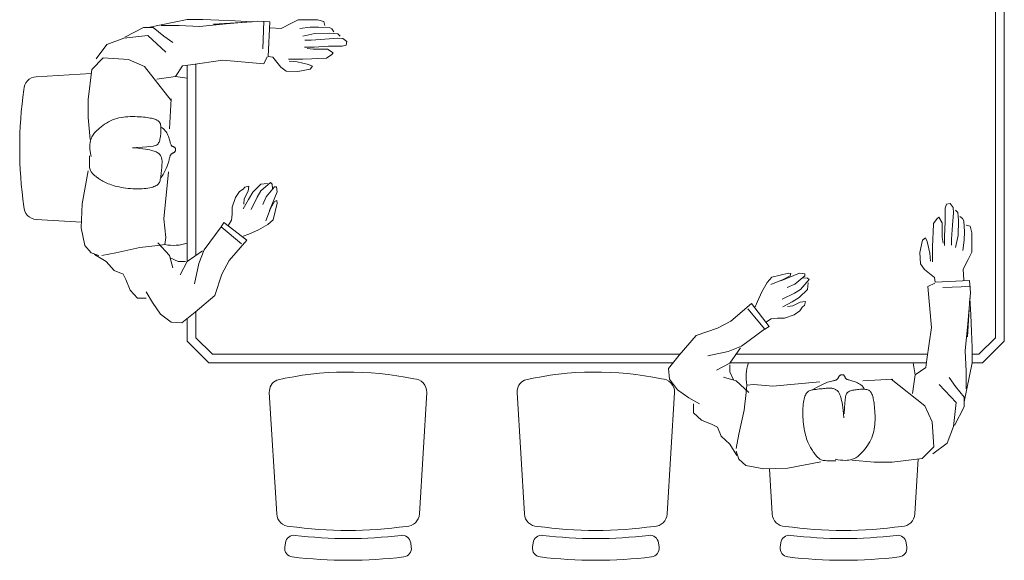
# Model space of a CAD drawing. Units: inches. Extents: x 1913 to 5309, y 1003 to 1733.
# Tile 17 of 23: x 4206 to 4274, y 1415 to 1452. Entities that reach past the tile are written whole.
import ezdxf

# ---------------------------------------------------------------- set-up
doc = ezdxf.new("R2010")
doc.units = ezdxf.units.IN
doc.layers.add('A-FURN', color=8, linetype='Continuous', lineweight=18)

# ---------------------------------------------------------------- blocks, each defined once
blk = doc.blocks.new('A$C421907B3')
for p, q in [((0.7245, 2.5796), (0.7652, 2.5876)), ((0.7652, 2.5876), (0.8209, 2.5856)), ((0.8209, 2.5856), (0.8965, 2.5714)), ((0.7017, 2.5468), (0.7079, 2.565)), ((0.7079, 2.565), (0.7245, 2.5796)), ((0.8897, 2.5609), (0.8883, 2.5594)), ((0.8911, 2.5623), (0.8897, 2.5609)), ((0.8926, 2.5635), (0.8911, 2.5623)), ((0.8941, 2.5647), (0.8926, 2.5635)), ((0.8958, 2.5657), (0.8941, 2.5647)), ((0.8976, 2.5665), (0.8958, 2.5657)), ((0.8996, 2.5672), (0.8976, 2.5665)), ((0.9018, 2.5678), (0.8996, 2.5672)), ((0.9043, 2.5682), (0.9018, 2.5678)), ((0.9071, 2.5684), (0.9043, 2.5682)), ((0.9102, 2.5686), (0.9071, 2.5684)), ((0.9137, 2.5687), (0.9102, 2.5686)), ((0.9175, 2.5687), (0.9137, 2.5687)), ((0.9217, 2.5687), (0.9175, 2.5687)), ((0.9264, 2.5687), (0.9217, 2.5687)), ((0.9314, 2.5687), (0.9264, 2.5687)), ((0.9361, 2.5662), (0.9297, 2.5647)), ((0.942, 2.5671), (0.9361, 2.5662)), ((0.9475, 2.5676), (0.942, 2.5671)), ((0.9525, 2.5677), (0.9475, 2.5676)), ((0.9571, 2.5675), (0.9525, 2.5677)), ((0.9614, 2.5669), (0.9571, 2.5675)), ((0.9652, 2.5662), (0.9614, 2.5669)), ((0.9686, 2.5653), (0.9652, 2.5662)), ((0.9684, 2.5672), (1.0195, 2.5715)), ((0.9717, 2.5643), (0.9686, 2.5653)), ((0.9745, 2.5632), (0.9717, 2.5643)), ((0.977, 2.5619), (0.9745, 2.5632)), ((0.9794, 2.5605), (0.977, 2.5619)), ((0.9818, 2.5588), (0.9794, 2.5605)), ((1.0195, 2.5715), (1.0607, 2.5715)), ((1.0607, 2.5715), (1.1301, 2.5633)), ((1.1301, 2.5633), (1.1567, 2.5368)), ((0.7038, 2.5568), (0.6875, 2.5302)), ((0.7017, 2.5405), (0.7079, 2.5077)), ((0.873, 2.5379), (0.8714, 2.5351)), ((0.8745, 2.5405), (0.873, 2.5379)), ((0.8761, 2.543), (0.8745, 2.5405)), ((0.8777, 2.5455), (0.8761, 2.543)), ((0.8792, 2.5478), (0.8777, 2.5455)), ((0.8808, 2.55), (0.8792, 2.5478)), ((0.8823, 2.5521), (0.8808, 2.55)), ((0.8839, 2.5541), (0.8823, 2.5521)), ((0.8853, 2.556), (0.8839, 2.5541)), ((0.8868, 2.5577), (0.8853, 2.556)), ((0.8883, 2.5594), (0.8868, 2.5577)), ((0.9841, 2.5568), (0.9818, 2.5588)), ((0.9865, 2.5545), (0.9841, 2.5568)), ((0.9891, 2.5519), (0.9865, 2.5545)), ((0.9918, 2.5489), (0.9891, 2.5519)), ((0.9948, 2.5455), (0.9918, 2.5489)), ((0.9978, 2.5419), (0.9948, 2.5455)), ((1.0008, 2.5379), (0.9978, 2.5419)), ((1.0037, 2.5338), (1.0008, 2.5379)), ((1.1546, 2.5531), (1.1875, 2.5285)), ((0.6875, 2.5302), (0.6672, 2.5117)), ((0.8641, 2.5181), (0.8628, 2.514)), ((0.8655, 2.522), (0.8641, 2.5181)), ((0.8669, 2.5256), (0.8655, 2.522)), ((0.8684, 2.5289), (0.8669, 2.5256)), ((0.8699, 2.5321), (0.8684, 2.5289)), ((0.8714, 2.5351), (0.8699, 2.5321)), ((1.0066, 2.5294), (1.0037, 2.5338)), ((1.0093, 2.5249), (1.0066, 2.5294)), ((1.0117, 2.5203), (1.0093, 2.5249)), ((1.0138, 2.5155), (1.0117, 2.5203)), ((1.0156, 2.5107), (1.0138, 2.5155)), ((1.1567, 2.5368), (1.153, 2.4792)), ((1.1875, 2.5285), (1.202, 2.4895)), ((0.6672, 2.5117), (0.6589, 2.4912)), ((0.7079, 2.5077), (0.7204, 2.4524)), ((0.8584, 2.4951), (0.8576, 2.49)), ((0.8594, 2.5001), (0.8584, 2.4951)), ((0.8604, 2.5049), (0.8594, 2.5001)), ((0.8616, 2.5096), (0.8604, 2.5049)), ((0.8628, 2.514), (0.8616, 2.5096)), ((1.0171, 2.5058), (1.0156, 2.5107)), ((1.0184, 2.5008), (1.0171, 2.5058)), ((1.0194, 2.4958), (1.0184, 2.5008)), ((1.0202, 2.4907), (1.0194, 2.4958)), ((0.6219, 2.4749), (0.6036, 2.4584)), ((0.6464, 2.4852), (0.6219, 2.4749)), ((0.6589, 2.4912), (0.6464, 2.4852)), ((0.8558, 2.474), (0.8554, 2.4686)), ((0.8562, 2.4794), (0.8558, 2.474)), ((0.8568, 2.4847), (0.8562, 2.4794)), ((0.8576, 2.49), (0.8568, 2.4847)), ((0.9491, 2.4609), (0.9498, 2.4698)), ((1.0208, 2.4855), (1.0202, 2.4907)), ((1.0212, 2.4802), (1.0208, 2.4855)), ((1.0214, 2.4749), (1.0212, 2.4802)), ((1.0215, 2.4696), (1.0214, 2.4749)), ((1.153, 2.4792), (1.1364, 2.4424)), ((1.202, 2.4895), (1.2083, 2.4342)), ((1.2041, 2.4875), (1.2266, 2.4445)), ((0.6036, 2.4584), (0.6036, 2.4379)), ((0.7204, 2.4524), (0.7246, 2.4114)), ((0.8552, 2.4632), (0.8551, 2.4579)), ((0.8551, 2.4579), (0.8552, 2.4527)), ((0.8554, 2.4686), (0.8552, 2.4632)), ((0.8552, 2.4527), (0.8554, 2.4476)), ((0.8554, 2.4476), (0.8557, 2.4428)), ((0.9474, 2.446), (0.9483, 2.453)), ((0.9483, 2.453), (0.9491, 2.4609)), ((0.9505, 2.4603), (0.9511, 2.447)), ((0.9511, 2.447), (0.9518, 2.4364)), ((1.0202, 2.4445), (1.0206, 2.4492)), ((1.0206, 2.4492), (1.021, 2.4541)), ((1.021, 2.4541), (1.0212, 2.4591)), ((1.0212, 2.4591), (1.0214, 2.4643)), ((1.0214, 2.4643), (1.0215, 2.4696)), ((0.6178, 2.4379), (0.5933, 2.4236)), ((0.8557, 2.4428), (0.8561, 2.4383)), ((0.8561, 2.4383), (0.8567, 2.4341)), ((0.8567, 2.4341), (0.8574, 2.4301)), ((0.8574, 2.4301), (0.8582, 2.4265)), ((0.8582, 2.4265), (0.8591, 2.4232)), ((0.9425, 2.4226), (0.9435, 2.426)), ((0.9435, 2.426), (0.9445, 2.43)), ((0.9445, 2.43), (0.9455, 2.4346)), ((0.9455, 2.4346), (0.9465, 2.4399)), ((0.9465, 2.4399), (0.9474, 2.446)), ((0.9518, 2.4364), (0.9526, 2.4283)), ((0.9526, 2.4283), (0.9535, 2.4222)), ((1.0168, 2.423), (1.0174, 2.4259)), ((1.0174, 2.4259), (1.0181, 2.429)), ((1.0181, 2.429), (1.0186, 2.4325)), ((1.0186, 2.4325), (1.0192, 2.4362)), ((1.0192, 2.4362), (1.0197, 2.4402)), ((1.0197, 2.4402), (1.0202, 2.4445)), ((1.1364, 2.4424), (1.0587, 2.3808)), ((1.2083, 2.4342), (1.1693, 2.3932)), ((1.2266, 2.4445), (1.2266, 2.422)), ((1.2447, 2.3435), (1.2266, 2.4332)), ((0.5667, 2.4051), (0.5484, 2.3805)), ((0.5933, 2.4236), (0.5667, 2.4051)), ((0.7308, 2.4114), (0.7018, 2.3846)), ((0.7246, 2.4114), (0.7267, 2.3949)), ((0.8591, 2.4232), (0.8601, 2.4202)), ((0.8601, 2.4202), (0.8612, 2.4176)), ((0.8612, 2.4176), (0.8624, 2.4152)), ((0.8624, 2.4152), (0.8637, 2.4132)), ((0.8637, 2.4132), (0.8651, 2.4114)), ((0.8651, 2.4114), (0.8666, 2.41)), ((0.8666, 2.41), (0.8682, 2.4088)), ((0.8682, 2.4088), (0.87, 2.4078)), ((0.87, 2.4078), (0.872, 2.407)), ((0.872, 2.407), (0.8742, 2.4063)), ((0.8742, 2.4063), (0.8767, 2.4058)), ((0.8767, 2.4058), (0.8794, 2.4052)), ((0.8794, 2.4052), (0.8824, 2.4048)), ((0.8801, 2.4042), (0.8884, 2.3992)), ((0.8824, 2.4048), (0.8857, 2.4043)), ((0.8857, 2.4043), (0.8891, 2.4039)), ((0.8891, 2.4039), (0.8925, 2.4035)), ((0.8925, 2.4035), (0.896, 2.4031)), ((0.896, 2.4031), (0.8995, 2.4027)), ((0.8995, 2.4027), (0.9028, 2.4024)), ((0.9028, 2.4024), (0.9059, 2.4022)), ((0.9059, 2.4022), (0.9088, 2.4019)), ((0.9088, 2.4019), (0.9114, 2.4018)), ((0.9114, 2.4018), (0.9138, 2.4016)), ((0.9182, 2.4016), (0.9201, 2.4017)), ((0.9201, 2.4017), (0.9219, 2.4019)), ((0.9219, 2.4019), (0.9237, 2.4022)), ((0.9237, 2.4022), (0.9254, 2.4026)), ((0.9254, 2.4026), (0.927, 2.4031)), ((0.927, 2.4031), (0.9286, 2.4037)), ((0.9286, 2.4037), (0.9301, 2.4044)), ((0.9301, 2.4044), (0.9315, 2.4052)), ((0.9315, 2.4052), (0.9329, 2.406)), ((0.9329, 2.406), (0.9341, 2.4069)), ((0.9341, 2.4069), (0.9353, 2.4079)), ((0.9353, 2.4079), (0.9363, 2.409)), ((0.9363, 2.409), (0.9373, 2.4102)), ((0.9373, 2.4102), (0.9382, 2.4116)), ((0.9382, 2.4116), (0.9391, 2.4131)), ((0.9391, 2.4131), (0.9399, 2.415)), ((0.9399, 2.415), (0.9408, 2.4171)), ((0.9408, 2.4171), (0.9416, 2.4196)), ((0.9416, 2.4196), (0.9425, 2.4226)), ((0.9535, 2.4222), (0.9546, 2.4177)), ((0.9546, 2.4177), (0.9558, 2.4146)), ((0.9558, 2.4146), (0.9572, 2.4124)), ((0.9572, 2.4124), (0.9588, 2.4109)), ((0.9588, 2.4109), (0.9606, 2.4096)), ((0.9606, 2.4096), (0.9626, 2.4086)), ((0.9626, 2.4086), (0.9647, 2.4077)), ((0.9647, 2.4077), (0.9671, 2.407)), ((0.9671, 2.407), (0.9696, 2.4064)), ((0.9696, 2.4064), (0.9722, 2.406)), ((0.9722, 2.406), (0.9751, 2.4055)), ((0.9751, 2.4055), (0.9781, 2.4052)), ((0.9781, 2.4052), (0.9812, 2.4048)), ((0.9812, 2.4048), (0.9844, 2.4045)), ((0.9844, 2.4045), (0.9877, 2.4043)), ((0.9877, 2.4043), (0.9909, 2.4041)), ((0.9909, 2.4041), (0.9941, 2.4041)), ((0.994, 2.3993), (0.9965, 2.4026)), ((0.9941, 2.4041), (0.9971, 2.4042)), ((0.9971, 2.4042), (0.9999, 2.4044)), ((0.9999, 2.4044), (1.0025, 2.4049)), ((1.0025, 2.4049), (1.0047, 2.4055)), ((1.0047, 2.4055), (1.0067, 2.4064)), ((1.0067, 2.4064), (1.0085, 2.4075)), ((1.0085, 2.4075), (1.01, 2.4087)), ((1.01, 2.4087), (1.0113, 2.4102)), ((1.0113, 2.4102), (1.0124, 2.4119)), ((1.0124, 2.4119), (1.0135, 2.4137)), ((1.0135, 2.4137), (1.0144, 2.4158)), ((1.0144, 2.4158), (1.0152, 2.418)), ((1.0152, 2.418), (1.016, 2.4204)), ((1.016, 2.4204), (1.0168, 2.423)), ((1.1077, 2.4136), (1.114, 2.3706)), ((1.2266, 2.422), (1.2062, 2.3974)), ((1.2308, 2.3624), (1.2308, 2.4035)), ((0.5484, 2.3805), (0.5463, 2.356)), ((0.7018, 2.3846), (0.6731, 2.3766)), ((0.6876, 2.3643), (0.6959, 2.3826)), ((0.7267, 2.3949), (0.7429, 2.3929)), ((0.7429, 2.3929), (0.7861, 2.3972)), ((0.7861, 2.3972), (0.8946, 2.387)), ((0.8884, 2.3992), (0.8957, 2.3952)), ((0.8957, 2.3952), (0.9019, 2.3921)), ((0.9019, 2.3921), (0.9073, 2.3897)), ((0.9073, 2.3897), (0.9119, 2.3881)), ((0.9119, 2.3881), (0.9157, 2.3869)), ((0.9138, 2.4016), (0.9161, 2.4016)), ((0.9157, 2.3869), (0.919, 2.386)), ((0.9161, 2.4016), (0.9182, 2.4016)), ((0.919, 2.386), (0.9217, 2.3854)), ((0.9217, 2.3854), (0.924, 2.3849)), ((0.924, 2.3849), (0.926, 2.3844)), ((0.926, 2.3844), (0.9277, 2.384)), ((0.9277, 2.384), (0.929, 2.3837)), ((0.929, 2.3837), (0.9302, 2.3833)), ((0.9302, 2.3833), (0.9312, 2.383)), ((0.9312, 2.383), (0.932, 2.3826)), ((0.932, 2.3826), (0.9327, 2.3823)), ((0.9327, 2.3823), (0.9334, 2.3818)), ((0.9334, 2.3818), (0.934, 2.3813)), ((0.934, 2.3813), (0.9346, 2.3808)), ((0.9346, 2.3808), (0.9351, 2.3803)), ((0.9351, 2.3803), (0.9356, 2.3797)), ((0.9356, 2.3797), (0.936, 2.379)), ((0.9533, 2.3785), (0.9536, 2.379)), ((0.9536, 2.379), (0.954, 2.3796)), ((0.954, 2.3796), (0.9546, 2.3801)), ((0.9546, 2.3801), (0.9554, 2.3805)), ((0.9554, 2.3805), (0.9564, 2.381)), ((0.9564, 2.381), (0.9577, 2.3815)), ((0.9577, 2.3815), (0.9593, 2.382)), ((0.9593, 2.382), (0.9611, 2.3826)), ((0.9611, 2.3826), (0.9632, 2.3832)), ((0.9632, 2.3832), (0.9655, 2.3838)), ((0.9655, 2.3838), (0.9679, 2.3845)), ((0.9679, 2.3845), (0.9705, 2.3853)), ((0.9705, 2.3853), (0.9731, 2.3861)), ((0.9731, 2.3861), (0.9757, 2.387)), ((0.9757, 2.387), (0.9784, 2.388)), ((0.9784, 2.388), (0.9811, 2.3892)), ((0.9811, 2.3892), (0.9837, 2.3905)), ((0.9837, 2.3905), (0.9863, 2.3922)), ((0.9863, 2.3922), (0.9889, 2.3941)), ((0.9889, 2.3941), (0.9915, 2.3965)), ((0.9915, 2.3965), (0.994, 2.3993)), ((0.9931, 2.3848), (1.0625, 2.3808)), ((1.2062, 2.3974), (1.1917, 2.3769)), ((0.6569, 2.3601), (0.6876, 2.3438)), ((0.6876, 2.3478), (0.6876, 2.3643)), ((0.936, 2.379), (0.9365, 2.3783)), ((0.9365, 2.3783), (0.9369, 2.3776)), ((0.9369, 2.3776), (0.9372, 2.3769)), ((0.9372, 2.3769), (0.9376, 2.3761)), ((0.9376, 2.3761), (0.938, 2.3753)), ((0.938, 2.3753), (0.9384, 2.3746)), ((0.9384, 2.3746), (0.9389, 2.3738)), ((0.9389, 2.3738), (0.9395, 2.3731)), ((0.9395, 2.3731), (0.9401, 2.3725)), ((0.9401, 2.3725), (0.9408, 2.3719)), ((0.9408, 2.3719), (0.9417, 2.3714)), ((0.9417, 2.3714), (0.9426, 2.371)), ((0.9426, 2.371), (0.9437, 2.3707)), ((0.9437, 2.3707), (0.9447, 2.3706)), ((0.9447, 2.3706), (0.9458, 2.3705)), ((0.9458, 2.3705), (0.9468, 2.3706)), ((0.9468, 2.3706), (0.9478, 2.3708)), ((0.9478, 2.3708), (0.9487, 2.3712)), ((0.9487, 2.3712), (0.9494, 2.3717)), ((0.9494, 2.3717), (0.9501, 2.3723)), ((0.9501, 2.3723), (0.9507, 2.3731)), ((0.9507, 2.3731), (0.9512, 2.3739)), ((0.9512, 2.3739), (0.9517, 2.3747)), ((0.9517, 2.3747), (0.9521, 2.3755)), ((0.9521, 2.3755), (0.9524, 2.3764)), ((0.9524, 2.3764), (0.9527, 2.3771)), ((0.9527, 2.3771), (0.953, 2.3778)), ((0.953, 2.3778), (0.9533, 2.3785)), ((1.114, 2.3706), (1.1095, 2.3436)), ((1.114, 2.3706), (1.1385, 2.3544)), ((1.2287, 2.3154), (1.2308, 2.3624)), ((0.5463, 2.356), (0.5709, 2.3252)), ((0.6876, 2.3438), (0.7122, 2.3088)), ((1.1385, 2.3544), (1.1406, 2.3358)), ((1.1406, 2.3358), (1.151, 2.262)), ((0.5709, 2.3252), (0.6099, 2.2802)), ((0.6835, 2.317), (0.6365, 2.3273)), ((0.7143, 2.3048), (0.6835, 2.317)), ((1.235, 2.2538), (1.2287, 2.3154)), ((0.7674, 2.2656), (0.7143, 2.3048)), ((0.6099, 2.2802), (0.659, 2.2637)), ((0.7288, 2.2187), (0.7675, 2.2658)), ((0.7675, 2.2658), (0.7779, 2.2598)), ((0.659, 2.2637), (0.6898, 2.2475)), ((0.6898, 2.2475), (0.7368, 2.2065)), ((0.7779, 2.2598), (0.7368, 2.2065)), ((0.7716, 2.2487), (0.7827, 2.2421)), ((1.151, 2.262), (1.1428, 2.1677)), ((1.2413, 2.1822), (1.235, 2.2538)), ((0.7827, 2.2421), (0.7969, 2.2406)), ((0.7969, 2.2406), (0.8131, 2.2406)), ((0.8131, 2.2406), (0.8354, 2.2325)), ((0.8354, 2.2325), (0.8487, 2.2236)), ((0.8487, 2.2236), (0.8546, 2.2147)), ((0.7509, 2.2021), (0.7458, 2.2146)), ((0.7606, 2.1798), (0.7509, 2.2021)), ((0.8094, 2.2146), (0.8309, 2.2028)), ((0.8324, 2.2124), (0.8198, 2.2132)), ((0.8309, 2.2028), (0.8472, 2.1925)), ((0.8494, 2.2036), (0.8324, 2.2124)), ((0.8613, 2.2021), (0.8494, 2.2036)), ((0.8546, 2.2147), (0.859, 2.211)), ((0.859, 2.211), (0.8613, 2.2021)), ((0.7732, 2.1583), (0.7606, 2.1798)), ((0.8079, 2.1969), (0.8361, 2.1828)), ((0.8361, 2.1828), (0.8502, 2.1747)), ((0.8472, 2.1925), (0.8658, 2.1747)), ((1.2392, 2.1535), (1.2413, 2.1822)), ((0.7835, 2.1457), (0.7732, 2.1583)), ((0.7814, 2.1628), (0.8102, 2.1517)), ((0.848, 2.1369), (0.805, 2.1547)), ((0.8191, 2.1695), (0.8369, 2.1621)), ((0.8369, 2.1621), (0.8599, 2.1429)), ((0.8502, 2.1747), (0.8695, 2.1518)), ((0.8658, 2.1747), (0.8672, 2.1591)), ((1.1428, 2.1677), (1.159, 2.1597)), ((1.1595, 2.1573), (1.158, 2.1467)), ((1.1595, 2.1573), (1.2392, 2.1535)), ((1.1777, 2.1697), (1.2413, 2.1677)), ((1.226, 2.1528), (1.2245, 2.1279)), ((0.8221, 2.1369), (0.7835, 2.1457)), ((0.8102, 2.1517), (0.8257, 2.1428)), ((0.828, 2.1376), (0.8221, 2.1369)), ((0.8257, 2.1428), (0.828, 2.1376)), ((0.8599, 2.1384), (0.848, 2.1369)), ((0.8658, 2.1481), (0.8561, 2.1473)), ((0.8599, 2.1429), (0.8599, 2.1384)), ((0.8695, 2.1518), (0.8658, 2.1481)), ((1.158, 2.1467), (1.1354, 2.1286)), ((1.1263, 2.1158), (1.1248, 2.0893)), ((1.1354, 2.1286), (1.1263, 2.1158)), ((1.1474, 2.0909), (1.149, 2.1089)), ((1.1535, 2.1105), (1.1536, 2.078)), ((1.2245, 2.1279), (1.2358, 2.1052)), ((1.1248, 2.0893), (1.1308, 2.0606)), ((1.1414, 2.0644), (1.1474, 2.0909)), ((1.2238, 2.0848), (1.2269, 2.0606)), ((1.2358, 2.1052), (1.2442, 2.0886)), ((1.2442, 2.0886), (1.2442, 2.0441)), ((1.1377, 2.0553), (1.1414, 2.0644)), ((1.1536, 2.078), (1.1543, 2.0568)), ((1.1762, 2.0539), (1.1784, 2.0674)), ((1.1815, 2.0735), (1.1815, 2.0516)), ((1.1974, 2.0584), (1.1974, 2.0727)), ((1.2064, 2.078), (1.2125, 2.0501)), ((1.1308, 2.0606), (1.1377, 2.0553)), ((1.1543, 2.0568), (1.1551, 2.0432)), ((1.1551, 2.0432), (1.1558, 2.0229)), ((1.1762, 2.0357), (1.1762, 2.0539)), ((1.1815, 2.0516), (1.1831, 2.0183)), ((1.1996, 2.0267), (1.1974, 2.0584)), ((1.2125, 2.0501), (1.2132, 2.0154)), ((1.2276, 2.0418), (1.2261, 2.0161)), ((1.2269, 2.0606), (1.2276, 2.0418)), ((1.2442, 2.0441), (1.2404, 2.029)), ((1.1558, 2.0229), (1.1641, 2.0108)), ((1.168, 2.0077), (1.1762, 2.0206)), ((1.1762, 2.0206), (1.1762, 2.0357)), ((1.1831, 2.0183), (1.1831, 1.9874)), ((1.2019, 1.9979), (1.1996, 2.0267)), ((1.2404, 2.029), (1.2314, 2.0267)), ((1.1641, 2.0108), (1.168, 2.0077)), ((1.2012, 1.9859), (1.2019, 1.9979)), ((1.2117, 1.9972), (1.2064, 1.9919)), ((1.2132, 2.0154), (1.2117, 1.9972)), ((1.223, 2.0108), (1.2163, 2.0063)), ((1.2261, 2.0161), (1.223, 2.0108)), ((1.1831, 1.9874), (1.186, 1.9783)), ((1.186, 1.9783), (1.1944, 1.9768)), ((1.1944, 1.9768), (1.2012, 1.9859)), ((0.3928, 1.2157), (0.4173, 1.234)), ((0.4173, 1.234), (0.4418, 1.2361)), ((0.4418, 1.2361), (0.4726, 1.2115)), ((0.3742, 1.1891), (0.3928, 1.2157)), ((0.4726, 1.2115), (0.5176, 1.1724)), ((0.3229, 1.1605), (0.3394, 1.1788)), ((0.3394, 1.1788), (0.36, 1.1787)), ((0.36, 1.1646), (0.3742, 1.1891)), ((0.3126, 1.1359), (0.3229, 1.1605)), ((0.5176, 1.1724), (0.5341, 1.1234)), ((0.3066, 1.1235), (0.3126, 1.1359)), ((0.4808, 1.0989), (0.4706, 1.1459)), ((0.2676, 1.0948), (0.2861, 1.1152)), ((0.2861, 1.1152), (0.3066, 1.1235)), ((0.4378, 1.1255), (0.454, 1.0947)), ((0.5341, 1.1234), (0.5503, 1.0926)), ((0.241, 1.0786), (0.2676, 1.0948)), ((0.4132, 1.0806), (0.4212, 1.1093)), ((0.4335, 1.0947), (0.4152, 1.0865)), ((0.45, 1.0947), (0.4335, 1.0947)), ((0.454, 1.0947), (0.489, 1.0702)), ((0.493, 1.0681), (0.4808, 1.0989)), ((0.5503, 1.0926), (0.5914, 1.0456)), ((0.2328, 1.0745), (0.2183, 1.0579)), ((0.2511, 1.0807), (0.2328, 1.0745)), ((0.2573, 1.0807), (0.2901, 1.0744)), ((0.2901, 1.0744), (0.3454, 1.062)), ((0.3864, 1.0516), (0.4132, 1.0806)), ((0.5322, 1.015), (0.493, 1.0681)), ((0.2183, 1.0579), (0.2102, 1.0171)), ((0.3454, 1.062), (0.3864, 1.0578)), ((0.3864, 1.0578), (0.4029, 1.0557)), ((0.4029, 1.0557), (0.4049, 1.0395)), ((0.5791, 1.0535), (0.532, 1.0149)), ((0.538, 1.0045), (0.5914, 1.0456)), ((0.4049, 1.0395), (0.4006, 0.9963)), ((0.5958, 1.0315), (0.5832, 1.0366)), ((0.618, 1.0218), (0.5958, 1.0315)), ((0.6395, 1.0092), (0.618, 1.0218)), ((0.2102, 1.0171), (0.2122, 0.9615)), ((0.532, 1.0149), (0.538, 1.0045)), ((0.5491, 1.0108), (0.5557, 0.9996)), ((0.5557, 0.9996), (0.5572, 0.9855)), ((0.635, 1.001), (0.6461, 0.9722)), ((0.6521, 0.9988), (0.6395, 1.0092)), ((0.6609, 0.9603), (0.6521, 0.9988)), ((0.4006, 0.9963), (0.4108, 0.8878)), ((0.5572, 0.9855), (0.5572, 0.9693)), ((0.6009, 0.9744), (0.615, 0.9462)), ((0.6609, 0.9344), (0.6432, 0.9774)), ((0.2122, 0.9615), (0.2264, 0.8858)), ((0.5572, 0.9693), (0.5653, 0.947)), ((0.5832, 0.9729), (0.595, 0.9515)), ((0.5854, 0.9499), (0.5846, 0.9626)), ((0.6283, 0.9633), (0.6357, 0.9455)), ((0.6461, 0.9722), (0.655, 0.9566)), ((0.655, 0.9566), (0.6602, 0.9544)), ((0.6602, 0.9544), (0.6609, 0.9603)), ((0.5653, 0.947), (0.5742, 0.9337)), ((0.5742, 0.9337), (0.5832, 0.9278)), ((0.5942, 0.933), (0.5854, 0.9499)), ((0.5957, 0.9211), (0.5942, 0.933)), ((0.595, 0.9515), (0.6053, 0.9352)), ((0.6053, 0.9352), (0.6232, 0.9166)), ((0.615, 0.9462), (0.6232, 0.9322)), ((0.6232, 0.9322), (0.6461, 0.9129)), ((0.6357, 0.9455), (0.655, 0.9225)), ((0.6594, 0.9225), (0.6609, 0.9344)), ((0.2548, 0.9063), (0.2573, 0.9078)), ((0.2573, 0.9078), (0.26, 0.9094)), ((0.26, 0.9094), (0.2628, 0.911)), ((0.2628, 0.911), (0.2657, 0.9125)), ((0.2657, 0.9125), (0.2689, 0.914)), ((0.2689, 0.914), (0.2723, 0.9155)), ((0.2723, 0.9155), (0.2759, 0.9169)), ((0.2759, 0.9169), (0.2797, 0.9183)), ((0.2797, 0.9183), (0.2839, 0.9196)), ((0.2839, 0.9196), (0.2883, 0.9208)), ((0.2883, 0.9208), (0.2929, 0.922)), ((0.2929, 0.922), (0.2977, 0.923)), ((0.2977, 0.923), (0.3027, 0.924)), ((0.3027, 0.924), (0.3078, 0.9248)), ((0.3078, 0.9248), (0.3131, 0.9255)), ((0.3131, 0.9255), (0.3184, 0.9261)), ((0.3184, 0.9261), (0.3238, 0.9266)), ((0.3238, 0.9266), (0.3293, 0.927)), ((0.3293, 0.927), (0.3347, 0.9272)), ((0.3347, 0.9272), (0.34, 0.9272)), ((0.34, 0.9272), (0.3452, 0.9272)), ((0.3452, 0.9272), (0.3502, 0.927)), ((0.3502, 0.927), (0.355, 0.9267)), ((0.355, 0.9267), (0.3595, 0.9262)), ((0.3595, 0.9262), (0.3638, 0.9257)), ((0.3638, 0.9257), (0.3677, 0.925)), ((0.3677, 0.925), (0.3713, 0.9242)), ((0.3713, 0.9242), (0.3746, 0.9233)), ((0.3746, 0.9233), (0.3776, 0.9223)), ((0.3776, 0.9223), (0.3803, 0.9212)), ((0.3803, 0.9212), (0.3826, 0.92)), ((0.3826, 0.92), (0.3847, 0.9187)), ((0.3847, 0.9187), (0.3864, 0.9173)), ((0.3864, 0.9173), (0.3878, 0.9158)), ((0.3878, 0.9158), (0.389, 0.9142)), ((0.389, 0.9142), (0.39, 0.9123)), ((0.39, 0.9123), (0.3908, 0.9104)), ((0.3908, 0.9104), (0.3915, 0.9081)), ((0.3915, 0.9081), (0.3921, 0.9057)), ((0.5832, 0.9278), (0.5869, 0.9233)), ((0.5869, 0.9233), (0.5957, 0.9211)), ((0.6232, 0.9166), (0.6387, 0.9151)), ((0.6461, 0.9129), (0.6498, 0.9166)), ((0.6498, 0.9166), (0.6506, 0.9263)), ((0.655, 0.9225), (0.6594, 0.9225)), ((0.2306, 0.8828), (0.2313, 0.8848)), ((0.2313, 0.8848), (0.2322, 0.8866)), ((0.2322, 0.8866), (0.2332, 0.8883)), ((0.2332, 0.8883), (0.2343, 0.8898)), ((0.2343, 0.8898), (0.2356, 0.8913)), ((0.2356, 0.8913), (0.237, 0.8927)), ((0.237, 0.8927), (0.2385, 0.8941)), ((0.2385, 0.8941), (0.2401, 0.8956)), ((0.2401, 0.8956), (0.2419, 0.897)), ((0.2419, 0.897), (0.2437, 0.8985)), ((0.2437, 0.8985), (0.2457, 0.9)), ((0.2457, 0.9), (0.2478, 0.9016)), ((0.2478, 0.9016), (0.25, 0.9031)), ((0.25, 0.9031), (0.2524, 0.9047)), ((0.2524, 0.9047), (0.2548, 0.9063)), ((0.3921, 0.9057), (0.3926, 0.903)), ((0.3926, 0.903), (0.3931, 0.8999)), ((0.3931, 0.8999), (0.3935, 0.8967)), ((0.3935, 0.8967), (0.394, 0.8933)), ((0.3936, 0.9023), (0.3986, 0.894)), ((0.394, 0.8933), (0.3944, 0.8898)), ((0.3944, 0.8898), (0.3947, 0.8863)), ((0.3947, 0.8863), (0.3951, 0.8829)), ((0.3986, 0.894), (0.4026, 0.8867)), ((0.4026, 0.8867), (0.4057, 0.8804)), ((0.2291, 0.8687), (0.2292, 0.8722)), ((0.2291, 0.8649), (0.2291, 0.8687)), ((0.2291, 0.8607), (0.2291, 0.8649)), ((0.2292, 0.8722), (0.2294, 0.8753)), ((0.2294, 0.8753), (0.2297, 0.8781)), ((0.2297, 0.8781), (0.2301, 0.8806)), ((0.2301, 0.8806), (0.2306, 0.8828)), ((0.3951, 0.8829), (0.3954, 0.8796)), ((0.3954, 0.8796), (0.3957, 0.8765)), ((0.3957, 0.8765), (0.3959, 0.8736)), ((0.3959, 0.8736), (0.3961, 0.871)), ((0.3961, 0.8623), (0.3959, 0.8604)), ((0.3961, 0.871), (0.3962, 0.8685)), ((0.3962, 0.8642), (0.3961, 0.8623)), ((0.3962, 0.8685), (0.3962, 0.8663)), ((0.3962, 0.8663), (0.3962, 0.8642)), ((0.4057, 0.8804), (0.4081, 0.8751)), ((0.4081, 0.8751), (0.4098, 0.8705)), ((0.4098, 0.8705), (0.411, 0.8667)), ((0.411, 0.8667), (0.4118, 0.8634)), ((0.4118, 0.8634), (0.4124, 0.8607)), ((0.2291, 0.856), (0.2291, 0.8607)), ((0.2291, 0.8509), (0.2291, 0.856)), ((0.2302, 0.8349), (0.2307, 0.8404)), ((0.2307, 0.8404), (0.2316, 0.8463)), ((0.2316, 0.8463), (0.2331, 0.8527)), ((0.3718, 0.8389), (0.3678, 0.8379)), ((0.3752, 0.8398), (0.3718, 0.8389)), ((0.3782, 0.8407), (0.3752, 0.8398)), ((0.3807, 0.8416), (0.3782, 0.8407)), ((0.3829, 0.8425), (0.3807, 0.8416)), ((0.3847, 0.8433), (0.3829, 0.8425)), ((0.3863, 0.8442), (0.3847, 0.8433)), ((0.3876, 0.8451), (0.3863, 0.8442)), ((0.3888, 0.846), (0.3876, 0.8451)), ((0.3899, 0.8471), (0.3888, 0.846)), ((0.3909, 0.8482), (0.3899, 0.8471)), ((0.3918, 0.8495), (0.3909, 0.8482)), ((0.3927, 0.8508), (0.3918, 0.8495)), ((0.3934, 0.8523), (0.3927, 0.8508)), ((0.3941, 0.8538), (0.3934, 0.8523)), ((0.3947, 0.8553), (0.3941, 0.8538)), ((0.3952, 0.857), (0.3947, 0.8553)), ((0.3956, 0.8587), (0.3952, 0.857)), ((0.3959, 0.8604), (0.3956, 0.8587)), ((0.4124, 0.8607), (0.4129, 0.8583)), ((0.4129, 0.8583), (0.4134, 0.8564)), ((0.4134, 0.8564), (0.4138, 0.8547)), ((0.4138, 0.8547), (0.4141, 0.8533)), ((0.4141, 0.8533), (0.4145, 0.8522)), ((0.4145, 0.8522), (0.4148, 0.8512)), ((0.4148, 0.8512), (0.4152, 0.8504)), ((0.4152, 0.8504), (0.4156, 0.8497)), ((0.4156, 0.8497), (0.416, 0.849)), ((0.416, 0.849), (0.4165, 0.8484)), ((0.4165, 0.8484), (0.417, 0.8478)), ((0.417, 0.8478), (0.4176, 0.8473)), ((0.4176, 0.8473), (0.4182, 0.8468)), ((0.4182, 0.8468), (0.4188, 0.8463)), ((0.4188, 0.8463), (0.4195, 0.8459)), ((0.4195, 0.8459), (0.4202, 0.8455)), ((0.4202, 0.8455), (0.4209, 0.8451)), ((0.4209, 0.8451), (0.4217, 0.8448)), ((0.4217, 0.8448), (0.4225, 0.8444)), ((0.4225, 0.8444), (0.4233, 0.8439)), ((0.4233, 0.8439), (0.424, 0.8435)), ((0.424, 0.8435), (0.4247, 0.8429)), ((0.4247, 0.8429), (0.4253, 0.8423)), ((0.4253, 0.8423), (0.4259, 0.8415)), ((0.4259, 0.8415), (0.4264, 0.8407)), ((0.4264, 0.8407), (0.4268, 0.8397)), ((0.4268, 0.8397), (0.4271, 0.8387)), ((0.4271, 0.8387), (0.4273, 0.8377)), ((0.2301, 0.8299), (0.2302, 0.8349)), ((0.2304, 0.8252), (0.2301, 0.8299)), ((0.2309, 0.821), (0.2304, 0.8252)), ((0.2316, 0.8172), (0.2309, 0.821)), ((0.2325, 0.8138), (0.2316, 0.8172)), ((0.3369, 0.8333), (0.328, 0.8326)), ((0.3448, 0.8341), (0.3369, 0.8333)), ((0.3375, 0.8319), (0.3508, 0.8313)), ((0.3518, 0.835), (0.3448, 0.8341)), ((0.3508, 0.8313), (0.3614, 0.8306)), ((0.3579, 0.8359), (0.3518, 0.835)), ((0.3632, 0.8369), (0.3579, 0.8359)), ((0.3614, 0.8306), (0.3695, 0.8298)), ((0.3678, 0.8379), (0.3632, 0.8369)), ((0.3695, 0.8298), (0.3757, 0.8289)), ((0.3757, 0.8289), (0.3801, 0.8278)), ((0.3801, 0.8278), (0.3832, 0.8265)), ((0.3832, 0.8265), (0.3854, 0.8251)), ((0.3854, 0.8251), (0.3869, 0.8235)), ((0.3869, 0.8235), (0.3882, 0.8218)), ((0.3882, 0.8218), (0.3892, 0.8198)), ((0.3892, 0.8198), (0.3901, 0.8176)), ((0.3901, 0.8176), (0.3908, 0.8153)), ((0.414, 0.8169), (0.4133, 0.8145)), ((0.4147, 0.8192), (0.414, 0.8169)), ((0.4152, 0.8213), (0.4147, 0.8192)), ((0.4158, 0.8231), (0.4152, 0.8213)), ((0.4163, 0.8247), (0.4158, 0.8231)), ((0.4168, 0.826), (0.4163, 0.8247)), ((0.4173, 0.827), (0.4168, 0.826)), ((0.4178, 0.8277), (0.4173, 0.827)), ((0.4183, 0.8283), (0.4178, 0.8277)), ((0.4188, 0.8288), (0.4183, 0.8283)), ((0.4194, 0.8291), (0.4188, 0.8288)), ((0.42, 0.8294), (0.4194, 0.8291)), ((0.4207, 0.8297), (0.42, 0.8294)), ((0.4215, 0.83), (0.4207, 0.8297)), ((0.4223, 0.8303), (0.4215, 0.83)), ((0.4231, 0.8307), (0.4223, 0.8303)), ((0.424, 0.8311), (0.4231, 0.8307)), ((0.4248, 0.8316), (0.424, 0.8311)), ((0.4255, 0.8322), (0.4248, 0.8316)), ((0.4261, 0.8329), (0.4255, 0.8322)), ((0.4267, 0.8337), (0.4261, 0.8329)), ((0.427, 0.8346), (0.4267, 0.8337)), ((0.4272, 0.8356), (0.427, 0.8346)), ((0.4273, 0.8366), (0.4272, 0.8356)), ((0.4273, 0.8377), (0.4273, 0.8366)), ((0.2306, 0.814), (0.2263, 0.7628)), ((0.2335, 0.8107), (0.2325, 0.8138)), ((0.2346, 0.8079), (0.2335, 0.8107)), ((0.2359, 0.8053), (0.2346, 0.8079)), ((0.2374, 0.8029), (0.2359, 0.8053)), ((0.2391, 0.8006), (0.2374, 0.8029)), ((0.241, 0.7983), (0.2391, 0.8006)), ((0.2433, 0.7958), (0.241, 0.7983)), ((0.246, 0.7933), (0.2433, 0.7958)), ((0.249, 0.7905), (0.246, 0.7933)), ((0.3908, 0.8153), (0.3914, 0.8128)), ((0.3914, 0.8128), (0.3919, 0.8101)), ((0.3919, 0.8101), (0.3923, 0.8073)), ((0.3923, 0.8073), (0.3926, 0.8043)), ((0.3926, 0.8043), (0.393, 0.8012)), ((0.393, 0.8012), (0.3933, 0.7979)), ((0.3933, 0.7979), (0.3936, 0.7947)), ((0.3936, 0.7947), (0.3937, 0.7915)), ((0.4037, 0.7935), (0.4014, 0.7909)), ((0.4057, 0.796), (0.4037, 0.7935)), ((0.4073, 0.7987), (0.4057, 0.796)), ((0.4087, 0.8013), (0.4073, 0.7987)), ((0.4098, 0.804), (0.4087, 0.8013)), ((0.4108, 0.8066), (0.4098, 0.804)), ((0.4117, 0.8093), (0.4108, 0.8066)), ((0.4126, 0.8119), (0.4117, 0.8093)), ((0.4133, 0.8145), (0.4126, 0.8119)), ((0.2523, 0.7876), (0.249, 0.7905)), ((0.256, 0.7846), (0.2523, 0.7876)), ((0.2599, 0.7816), (0.256, 0.7846)), ((0.264, 0.7786), (0.2599, 0.7816)), ((0.2684, 0.7758), (0.264, 0.7786)), ((0.2729, 0.7731), (0.2684, 0.7758)), ((0.2776, 0.7707), (0.2729, 0.7731)), ((0.2823, 0.7686), (0.2776, 0.7707)), ((0.3876, 0.7711), (0.386, 0.7699)), ((0.3891, 0.7724), (0.3876, 0.7711)), ((0.3904, 0.7739), (0.3891, 0.7724)), ((0.3914, 0.7756), (0.3904, 0.7739)), ((0.3923, 0.7776), (0.3914, 0.7756)), ((0.393, 0.7799), (0.3923, 0.7776)), ((0.3934, 0.7825), (0.393, 0.7799)), ((0.3937, 0.7853), (0.3934, 0.7825)), ((0.3937, 0.7915), (0.3938, 0.7883)), ((0.3938, 0.7883), (0.3937, 0.7853)), ((0.3986, 0.7884), (0.3953, 0.7859)), ((0.4014, 0.7909), (0.3986, 0.7884)), ((0.413, 0.7893), (0.417, 0.7199)), ((0.2263, 0.7628), (0.2263, 0.7217)), ((0.2871, 0.7668), (0.2823, 0.7686)), ((0.292, 0.7652), (0.2871, 0.7668)), ((0.297, 0.764), (0.292, 0.7652)), ((0.302, 0.7629), (0.297, 0.764)), ((0.3071, 0.7621), (0.302, 0.7629)), ((0.3123, 0.7616), (0.3071, 0.7621)), ((0.3176, 0.7612), (0.3123, 0.7616)), ((0.3229, 0.7609), (0.3176, 0.7612)), ((0.3282, 0.7609), (0.3229, 0.7609)), ((0.3335, 0.7609), (0.3282, 0.7609)), ((0.3387, 0.7611), (0.3335, 0.7609)), ((0.3438, 0.7614), (0.3387, 0.7611)), ((0.3486, 0.7618), (0.3438, 0.7614)), ((0.3533, 0.7622), (0.3486, 0.7618)), ((0.3576, 0.7627), (0.3533, 0.7622)), ((0.3617, 0.7632), (0.3576, 0.7627)), ((0.3654, 0.7637), (0.3617, 0.7632)), ((0.3688, 0.7643), (0.3654, 0.7637)), ((0.3719, 0.7649), (0.3688, 0.7643)), ((0.3748, 0.7656), (0.3719, 0.7649)), ((0.3774, 0.7663), (0.3748, 0.7656)), ((0.3799, 0.7671), (0.3774, 0.7663)), ((0.3821, 0.768), (0.3799, 0.7671)), ((0.3841, 0.7689), (0.3821, 0.768)), ((0.386, 0.7699), (0.3841, 0.7689)), ((0.2263, 0.7217), (0.2345, 0.6523)), ((0.3554, 0.646), (0.417, 0.7237)), ((0.3842, 0.6746), (0.4272, 0.6684)), ((0.4272, 0.6684), (0.4542, 0.6729)), ((0.4272, 0.6684), (0.4435, 0.6438)), ((0.6821, 0.6561), (0.7085, 0.6576)), ((0.7085, 0.6576), (0.7372, 0.6515)), ((0.2345, 0.6523), (0.261, 0.6256)), ((0.3186, 0.6294), (0.3554, 0.646)), ((0.4435, 0.6438), (0.462, 0.6418)), ((0.462, 0.6418), (0.5358, 0.6313)), ((0.5358, 0.6313), (0.6302, 0.6396)), ((0.6302, 0.6396), (0.6381, 0.6233)), ((0.6511, 0.6244), (0.6692, 0.647)), ((0.6692, 0.647), (0.6821, 0.6561)), ((0.707, 0.6349), (0.6889, 0.6334)), ((0.7335, 0.6409), (0.707, 0.6349)), ((0.7425, 0.6447), (0.7335, 0.6409)), ((0.7372, 0.6515), (0.7425, 0.6447)), ((0.2448, 0.6277), (0.2693, 0.5949)), ((0.261, 0.6256), (0.3186, 0.6294)), ((0.3636, 0.5741), (0.4047, 0.6131)), ((0.6405, 0.6229), (0.6511, 0.6244)), ((0.6405, 0.6229), (0.6444, 0.5432)), ((0.6873, 0.6288), (0.7199, 0.6288)), ((0.7199, 0.6288), (0.741, 0.6281)), ((0.741, 0.6281), (0.7546, 0.6273)), ((0.7546, 0.6273), (0.775, 0.6265)), ((0.775, 0.6265), (0.787, 0.6183)), ((0.7901, 0.6144), (0.7772, 0.6062)), ((0.787, 0.6183), (0.7901, 0.6144)), ((0.2693, 0.5949), (0.3083, 0.5804)), ((0.4004, 0.5761), (0.4209, 0.5906)), ((0.6281, 0.6047), (0.6301, 0.5411)), ((0.7243, 0.6009), (0.7462, 0.6009)), ((0.744, 0.6062), (0.7304, 0.6039)), ((0.7621, 0.6062), (0.744, 0.6062)), ((0.7462, 0.6009), (0.7795, 0.5993)), ((0.7772, 0.6062), (0.7621, 0.6062)), ((0.7795, 0.5993), (0.8105, 0.5993)), ((0.8105, 0.5993), (0.8195, 0.5963)), ((0.8195, 0.5963), (0.8211, 0.588)), ((0.3083, 0.5804), (0.3636, 0.5741)), ((0.3103, 0.5783), (0.3533, 0.5558)), ((0.3759, 0.5558), (0.4004, 0.5761)), ((0.7198, 0.576), (0.7477, 0.5699)), ((0.7395, 0.585), (0.7251, 0.585)), ((0.7712, 0.5828), (0.7395, 0.585)), ((0.7477, 0.5699), (0.7825, 0.5691)), ((0.7999, 0.5804), (0.7712, 0.5828)), ((0.7825, 0.5691), (0.8006, 0.5707)), ((0.8119, 0.5812), (0.7999, 0.5804)), ((0.8006, 0.5707), (0.8059, 0.576)), ((0.8211, 0.588), (0.8119, 0.5812)), ((0.3533, 0.5558), (0.3759, 0.5558)), ((0.4543, 0.5377), (0.3646, 0.5558)), ((0.4354, 0.5516), (0.3944, 0.5516)), ((0.4825, 0.5536), (0.4354, 0.5516)), ((0.544, 0.5474), (0.4825, 0.5536)), ((0.6156, 0.5411), (0.544, 0.5474)), ((0.645, 0.5564), (0.6699, 0.5579)), ((0.6699, 0.5579), (0.6926, 0.5466)), ((0.6926, 0.5466), (0.7092, 0.5382)), ((0.713, 0.5586), (0.7372, 0.5555)), ((0.7372, 0.5555), (0.756, 0.5548)), ((0.756, 0.5548), (0.7817, 0.5563)), ((0.7689, 0.5419), (0.7711, 0.551)), ((0.7817, 0.5563), (0.787, 0.5593)), ((0.787, 0.5593), (0.7916, 0.5661)), ((0.6444, 0.5432), (0.6156, 0.5411)), ((0.7092, 0.5382), (0.7538, 0.5382)), ((0.7538, 0.5382), (0.7689, 0.5419))]:
    blk.add_line(p, q)
at = {"ltscale": 0.1}
for points in [[(0.7784, 2.5871), (0.7847, 2.6911, -0.399285), (0.8147, 2.7196, -0.071734), (1.0831, 2.7196, -0.399285), (1.1131, 2.6911), (1.1208, 2.5644)], [(0.2107, 1.004), (0.1067, 0.9977, 0.399285), (0.0782, 0.9677, 0.071734), (0.0782, 0.6992, 0.399285), (0.1067, 0.6693), (0.2334, 0.6616)]]:
    blk.add_lwpolyline(points, format="xyb", dxfattribs=at)
for points in [[(0.4542, 1.2262), (0.4542, 2.2936), (0.5042, 2.3436), (0.5562, 2.3436)], [(0.6878, 2.3436), (1.1397, 2.3436)], [(0.4742, 1.2101), (0.4742, 2.2853), (0.5125, 2.3236), (0.5723, 2.3236)], [(0.7018, 2.3236), (1.1423, 2.3236)], [(0.4542, 0.6426), (0.4542, 1.0946)], [(0.4742, 0.64), (0.4742, 1.0806)], [(1.3342, 0.5966), (1.3342, 0.5218), (1.2959, 0.4835), (0.5125, 0.4835), (0.4742, 0.5218), (0.4742, 0.5375)], [(1.3542, 0.5878), (1.3542, 0.5135), (1.3042, 0.4635), (0.5042, 0.4635), (0.4542, 0.5135), (0.4542, 0.5377)]]:
    blk.add_lwpolyline(points, dxfattribs=at)
for points in [[(1.2332, 2.2712), (1.2341, 2.2831), (1.2396, 2.1946), (1.2396, 2.1946), (1.2419, 2.2332), (1.2437, 2.2711), (1.2448, 2.3081), (1.2452, 2.3436)], [(0.5267, 0.5491), (0.5148, 0.5482), (0.6033, 0.5427), (0.6033, 0.5427), (0.5647, 0.5405), (0.5267, 0.5387), (0.4898, 0.5376), (0.4542, 0.5371)]]:
    blk.add_lwpolyline(points)
for points in [[(0.0782, 2.1079, -0.399285), (0.1067, 2.1378), (0.3861, 2.1548, -0.305593), (0.4148, 2.1375, -0.109362), (0.4176, 1.8225, -0.429301), (0.3861, 1.7925), (0.1067, 1.8094, -0.399285), (0.0782, 1.8394, -0.071734)], [(0.05, 1.9736, 0.030867), (0.0575, 1.8517, -0.408428), (0.0405, 1.8294), (0.0306, 1.828, -0.419966), (0.0079, 1.8453, -0.030916), (0, 1.9736, -0.030916), (0.0079, 2.1019, -0.419966), (0.0306, 2.1193), (0.0405, 2.1178, -0.408428), (0.0575, 2.0956, 0.030867)], [(0.0782, 1.5378, -0.399285), (0.1067, 1.5678), (0.3861, 1.5847, -0.305593), (0.4148, 1.5674, -0.109362), (0.4176, 1.2524, -0.429301), (0.3861, 1.2224), (0.1067, 1.2393, -0.399285), (0.0782, 1.2693, -0.071734)], [(0.05, 1.4036, 0.030867), (0.0575, 1.2816, -0.408428), (0.0405, 1.2593), (0.0306, 1.2579, -0.419966), (0.0079, 1.2752, -0.030916), (0, 1.4036, -0.030916), (0.0079, 1.5319, -0.419966), (0.0306, 1.5492), (0.0405, 1.5478, -0.408428), (0.0575, 1.5255, 0.030867)], [(0.05, 0.8335, -0.030867), (0.0575, 0.9554, 0.408428), (0.0405, 0.9777), (0.0306, 0.9791, 0.419966), (0.0079, 0.9618, 0.030916), (0, 0.8335, 0.030916), (0.0079, 0.7052, 0.419966), (0.0306, 0.6878), (0.0405, 0.6893, 0.408428), (0.0575, 0.7115, -0.030867)]]:
    blk.add_lwpolyline(points, format="xyb", close=True, dxfattribs=at)
for centre, start, end in [((0.8297, 2.3756), 169.4107, 197.7809), ((0.4222, 0.9527), 72.2191, 100.5893)]:
    blk.add_arc(centre, 0.1048, start, end)

msp = doc.modelspace()

# ---------------------------------------------------------------- block references
at = {"layer": 'A-FURN', "xscale": 30.26057373645948, "yscale": 30.26057373645948, "zscale": 30.26057373645948, "rotation": 89.99999999999996}
msp.add_blockref('A$C421907B3', (4288.218, 1414.678), dxfattribs=at)

doc.saveas('drawing.dxf')
